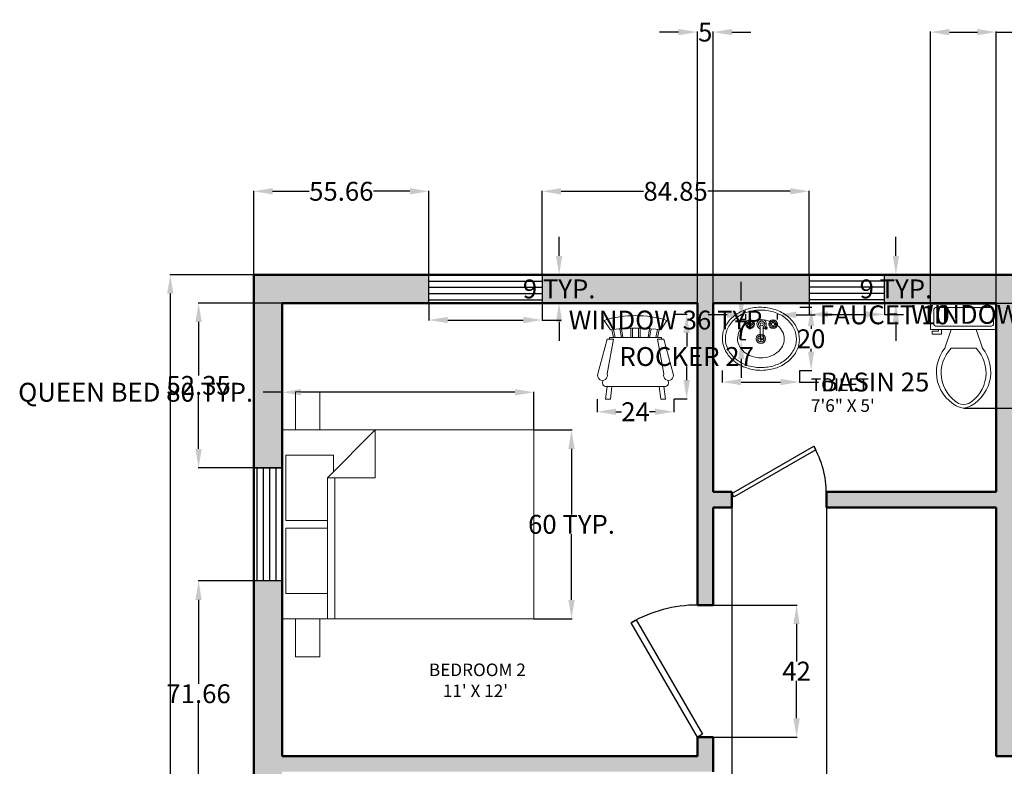
# Model space of a CAD drawing. Units: inches. Extents: x -40 to 482, y -490 to 102.
# Tile 3 of 4: x -40 to 273, y -136 to 102. Entities that reach past the tile are written whole.
import ezdxf

# ---------------------------------------------------------------- set-up
doc = ezdxf.new("R2010")
doc.units = ezdxf.units.IN
doc.header["$MEASUREMENT"] = 0
for name, color, linetype, lineweight in [('A-ANNO-DIMS', 2, 'Continuous', 18), ('A-AREA-IDEN', 7, 'Continuous', 18), ('A-FLOR-FIXT', 9, 'Continuous', 18), ('A-FURN', 8, 'Continuous', 18), ('A-WALL', 7, 'Continuous', 50), ('A-WALL-PATT', 251, 'Continuous', 13), ('DOOR', 21, 'Continuous', 25), ('WINDOW', 151, 'Continuous', 25)]:
    doc.layers.add(name, color=color, linetype=linetype, lineweight=lineweight)
doc.styles.get("Standard").update_dxf_attribs({"font": 'arial.ttf'})
doc.dimstyles.get("Standard").update_dxf_attribs({"dimtxt": 6, "dimasz": 6, "dimexe": 0.18, "dimexo": 0.0625, "dimgap": 0.09, "dimtad": 0, "dimtih": 1, "dimtoh": 1, "dimdec": 3, "dimzin": 0, "dimdsep": 46, "dimlunit": 4, "dimtxsty": 'Standard', "dimcen": 0.09, "dimadec": 0, "dimazin": 0, "dimtfac": 1, "dimtdec": 3, "dimtofl": 0, "dimtmove": 0, "dimatfit": 3, "dimfxl": 1, "dimtolj": 1, "dimtzin": 0, "dimarcsym": 0})

# ---------------------------------------------------------------- blocks, each defined once
blk = doc.blocks.new('*U2')
for p, q in [((0, 0), (0, -6)), ((40, 0), (40, -6))]:
    blk.add_line(p, q)
blk.add_lwpolyline([(0, 0), (34.64, 20), (35.52, 18.48), (0.87, -1.52)], close=True)
blk.add_arc((0, 0), 40, 0, 30)
blk = doc.blocks.new('*U3')
for p, q in [((-40, 0), (-40, 6)), ((0, 0), (0, 6))]:
    blk.add_line(p, q)
blk.add_lwpolyline([(0, 0), (-34.64, -20), (-35.52, -18.48), (-0.88, 1.52)], close=True)
blk.add_arc((0, 0), 40, 180, 210)
blk = doc.blocks.new('WINDOW')
for p, q in [((0, 0), (36, 0)), ((0, -9), (0, 0)), ((36, 0), (36, -9)), ((0, -2), (36, -2)), ((0, -4), (36, -4)), ((0, -6), (36, -6)), ((0, -8), (36, -8)), ((36, -9), (0, -9))]:
    blk.add_line(p, q)
blk = doc.blocks.new('Bed - Queen')
for p, q in [((0, -80.00003), (0, 0)), ((0, 0), (59.99999, 0)), ((59.99999, 0), (59.99999, -80.00003)), ((7.99999, -1.2), (28.79998, -1.2)), ((7.99999, -14.4), (7.99999, -1.2)), ((28.79998, -1.2), (28.79998, -14.4)), ((31.19999, -1.2), (51.99999, -1.2)), ((31.19999, -14.4), (31.19999, -1.2)), ((51.99999, -1.2), (51.99999, -16.4)), ((0, -14.4), (44.8, -14.4)), ((59.99999, -29.6), (44.8, -14.4)), ((44.8, -14.4), (44.8, -29.6)), ((44.8, -16.8), (0, -16.8)), ((51.99999, -16.4), (46.79936, -16.4)), ((44.8, -29.6), (59.99999, -29.6)), ((59.99999, -80.00003), (0, -80.00003))]:
    blk.add_line(p, q)
blk = doc.blocks.new('*U13')
for p, q in [((9.5, -6), (9.5, -2)), ((-10, -8.5), (-8, -8.5)), ((-10, -9.5), (-10, -8.5)), ((-8, -8.5), (-8, -8)), ((-7, -8), (-7, -9.5)), ((-4, -8), (-6, -14)), ((4, -8), (6, -14)), ((-7, -9.5), (-10, -9.5)), ((4, -14), (-4, -14))]:
    blk.add_line(p, q)
blk.add_lwpolyline([(10.5, -8), (10.5, 0), (-10.5, 0), (-10.5, -8)], close=True)
for points in [[(-9.5, -2), (-9.5, -6)], [(8.5, -1), (-8.5, -1)], [(-8.5, -7), (8.5, -7)]]:
    blk.add_lwpolyline(points)
for centre, radius, start, end in [((-8.62, -1.88), 0.884, 81.8699, 188.1301), ((8.62, -1.88), 0.884, 351.8699, 98.1301), ((-8.62, -6.12), 0.884, 171.8699, 278.1301), ((8.62, -6.12), 0.884, 261.8699, 8.1301), ((3.52, -21.58), 12.17, 141.4691, 247.9714), ((4.2, -21.82), 11.33, 136.3677, 238.9468), ((-3.52, -21.58), 12.17, 292.0284, 38.5307), ((-4.2, -21.82), 11.33, 301.053, 43.6321), ((0, -27.88), 4, 245.7318, 294.2682), ((0, -29), 4, 254.8605, 285.1395)]:
    blk.add_arc(centre, radius, start, end)
blk = doc.blocks.new('Chair - Rocking')
for p, q in [((-8, -4.5), (-10, -1.5)), ((8, -4.5), (10, -1.5)), ((-7.5, -4.5), (-7, -7)), ((-6.5, -7), (-7.02225, -4.43)), ((-4.5, -7), (-4.96674, -4.19951)), ((-4, -7), (-4.40532, -4.16272)), ((-1.5, -4.05012), (-1.5, -7)), ((-1, -7), (-1, -4.05012)), ((1, -7), (1, -4.04655)), ((1.5, -4.05012), (1.5, -7)), ((4, -7), (4.40187, -4.18694)), ((4.5, -7), (4.96761, -4.19437)), ((6.5, -7), (7, -4.4057)), ((7.5, -4.5), (7, -7)), ((-9, -7.5), (-12, -18.49999)), ((-7, -7.5), (-9, -7.5)), ((-9, -18.49999), (-7, -7.5)), ((-8.23428, -6.99939), (-8.3093, -7.47958)), ((-8.23041, -7), (8.23915, -7)), ((7, -7.5), (9, -7.5)), ((9, -18.49999), (7, -7.5)), ((8.31071, -7.48854), (8.23449, -7.00073)), ((9, -7.5), (12, -18.49999)), ((-10.36644, -20.64523), (-10.5, -21.49999)), ((10.5, -21.49999), (10.3575, -20.58798)), ((-9, -22.49999), (-9.5, -26.49999)), ((0, -22.49999), (-9.5, -22.49999)), ((-8, -26.49999), (-7.5, -22.49999)), ((0, -22.49999), (9.5, -22.49999)), ((8, -26.49999), (7.5, -22.49999)), ((9, -22.49999), (9.5, -26.49999)), ((-9.5, -26.49999), (-8, -26.49999)), ((9.5, -26.49999), (8, -26.49999))]:
    blk.add_line(p, q)
for centre, radius, start, end in [((0, -34.08333), 34.08333, 72.93847, 107.0615), ((0, -68.25004), 64.25, 93.92211, 97.15267), ((0, -68.25004), 64.25, 82.84733, 93.92211), ((-10.5, -18.99999), 1.58114, 161.5651, 18.43495), ((10.5, -18.99999), 1.58114, 161.5651, 18.43495), ((-9.5, -21.49999), 1, 180, 270), ((9.5, -21.49999), 1, 270, 0)]:
    blk.add_arc(centre, radius, start, end)
blk = doc.blocks.new('Sink - Oval top')
for p, q in [((-1, 0), (1, 0)), ((0, 1), (0, -1))]:
    blk.add_line(p, q)
for points in [[(-12.23, 0.39, 0.117634), (-11.46, -3.36, 0.104469), (-8.88, -6.8, 0.090016), (-5.08, -9.07, 0.08192), (-0.32, -10.02, 0.08192), (4.49, -9.38, 0.090016), (8.42, -7.36, 0.104469), (11.22, -4.09, 0.117634), (12.23, -0.39, 0.117634), (11.46, 3.36, 0.104469), (8.88, 6.8, 0.090016), (5.08, 9.07, 0.08192), (0.32, 10.02, 0.08192), (-4.49, 9.38, 0.090016), (-8.42, 7.36, 0.104469), (-11.22, 4.09, 0.117634)], [(-11.29, 0.16, 0.118622), (-10.52, -3.25, 0.104678), (-8.07, -6.36, 0.089562), (-4.54, -8.37, 0.081185), (-0.13, -9.15, 0.081185), (4.3, -8.49, 0.089562), (7.89, -6.58, 0.104678), (10.42, -3.55, 0.118622), (11.29, -0.16, 0.118622), (10.52, 3.25, 0.104678), (8.07, 6.36, 0.089562), (4.54, 8.37, 0.081185), (0.13, 9.15, 0.081185), (-4.3, 8.49, 0.089562), (-7.89, 6.58, 0.104678), (-10.42, 3.55, 0.118622)], [(-7.42, 0.08, 0.118283), (-6.91, -2.17, 0.104607), (-5.29, -4.21, 0.089718), (-2.97, -5.53, 0.081436), (-0.07, -6.04, 0.081436), (2.84, -5.59, 0.089718), (5.2, -4.33, 0.104607), (6.86, -2.32, 0.118283), (7.42, -0.08, 0.118283), (6.91, 2.17, 0.104607), (5.29, 4.21, 0.089718), (2.97, 5.53, 0.081436), (0.07, 6.04, 0.081436), (-2.84, 5.59, 0.089718), (-5.2, 4.33, 0.104607), (-6.86, 2.32, 0.118283)]]:
    blk.add_lwpolyline(points, format="xyb", close=True)
for radius in [1.5, 1]:
    blk.add_circle((0, 0), radius)
blk = doc.blocks.new('Faucet - Bathroom top')
for p, q in [((-4.107, 0.125), (-4.375, 0.125)), ((-3.75, 0.4788), (-3.75, 0.75)), ((-3.5, 0.482), (-3.5, 0.75)), ((-3.1461, 0.125), (-2.875, 0.125)), ((3.143, 0.125), (2.875, 0.125)), ((3.5, 0.4788), (3.5, 0.75)), ((3.75, 0.482), (3.75, 0.75)), ((4.1039, 0.125), (4.375, 0.125)), ((-4.1039, -0.125), (-4.375, -0.125)), ((-3.75, -0.4821), (-3.75, -0.75)), ((-3.5, -0.4789), (-3.5, -0.75)), ((-3.143, -0.125), (-2.875, -0.125)), ((-0.5, -0.8639), (-0.5, -4.5)), ((0.5, -4.5), (0.5, -0.8631)), ((3.1461, -0.125), (2.875, -0.125)), ((3.5, -0.4821), (3.5, -0.75)), ((3.75, -0.4789), (3.75, -0.75)), ((4.107, -0.125), (4.375, -0.125))]:
    blk.add_line(p, q)
for centre, radius in [((-3.625, 0), 1.375), ((-4.625, 0), 0.2795), ((-3.625, 0), 0.5), ((-3.625, 1), 0.2795), ((-2.625, 0), 0.2795), ((0, 0), 0.5), ((3.625, 0), 1.375), ((2.625, 0), 0.2795), ((3.625, 0), 0.5), ((3.625, 1), 0.2795), ((4.625, 0), 0.2795), ((-3.625, -1), 0.2795), ((3.625, -1), 0.2795)]:
    blk.add_circle(centre, radius)
for centre, radius, start, end in [((-3.625, 0), 1, 105.2407, 164.2093), ((-3.625, 0), 1, 16.44125, 74.07887), ((0, 0), 1.5, 289.6514, 250.3603), ((0, 0), 1, 300.3431, 239.7554), ((3.625, 0), 1, 106.12, 164.0884), ((3.625, 0), 1, 16.23422, 73.90469), ((-3.625, 0), 1, 196.2342, 253.9047), ((-3.625, 0), 1, 286.12, 344.0884), ((3.625, 0), 1, 196.4413, 254.0789), ((3.625, 0), 1, 285.2407, 344.2093), ((0, -4.5), 0.5, 180, 0)]:
    blk.add_arc(centre, radius, start, end)
blk = doc.blocks.new('WIN-24IN')
for p, q in [((24, 9), (0, 9)), ((0, 9), (0, 0)), ((24, 7), (0, 7)), ((24, 0), (24, 9)), ((24, 5), (0, 5)), ((24, 3), (0, 3)), ((24, 1), (0, 1)), ((0, 0), (24, 0))]:
    blk.add_line(p, q)
blk = doc.blocks.new('NIGHTSTAND')
blk.add_lwpolyline([(0, 12.15), (7.78, 12.15), (7.78, 0), (0, 0)], close=True)
blk = doc.blocks.new('*D24')
at = {"layer": 'A-ANNO-DIMS', "color": 0, "lineweight": -2, "transparency": 16777216}
for p, q in [((90.52, 11.43), (90.52, 5.91)), ((126.52, 11.43), (126.52, 5.91)), ((96.52, 6.09), (120.52, 6.09)), ((126.52, 6.09), (132.52, 6.09))]:
    blk.add_line(p, q, dxfattribs=at)
at = {"layer": 'A-ANNO-DIMS', "color": 0, "transparency": 16777216}
for points in [[(96.52, 7.09), (96.52, 5.09), (90.52, 6.09)], [(120.52, 7.09), (120.52, 5.09), (126.52, 6.09)]]:
    blk.add_solid(points, dxfattribs=at)
at = {"layer": 'Defpoints', "color": 0, "transparency": 16777216}
for p in [(90.52, 11.49), (126.52, 11.49), (126.52, 6.09)]:
    blk.add_point(p, dxfattribs=at)
at = {"layer": 'A-ANNO-DIMS', "color": 0, "transparency": 16777216, "insert": (166.89, 6.09), "char_height": 6, "attachment_point": 5}
blk.add_mtext('\\A1;WINDOW 36 TYP.', dxfattribs=at)
blk = doc.blocks.new('*D25')
at = {"layer": 'A-ANNO-DIMS', "color": 0, "lineweight": -2, "transparency": 16777216}
for p, q in [((131.92, 26.49), (131.92, 32.49)), ((126.58, 20.49), (132.1, 20.49)), ((126.58, 11.49), (132.1, 11.49)), ((131.92, 5.49), (131.92, -0.51))]:
    blk.add_line(p, q, dxfattribs=at)
at = {"layer": 'A-ANNO-DIMS', "color": 0, "transparency": 16777216}
for points in [[(130.92, 26.49), (132.92, 26.49), (131.92, 20.49)], [(130.92, 5.49), (132.92, 5.49), (131.92, 11.49)]]:
    blk.add_solid(points, dxfattribs=at)
at = {"layer": 'Defpoints', "color": 0, "transparency": 16777216}
for p in [(126.52, 20.49), (131.92, 20.49), (126.52, 11.49)]:
    blk.add_point(p, dxfattribs=at)
at = {"layer": 'A-ANNO-DIMS', "color": 0, "transparency": 16777216, "insert": (131.92, 15.99), "char_height": 6, "attachment_point": 5}
blk.add_mtext('\\A1;9 TYP.', dxfattribs=at)
blk = doc.blocks.new('*D26')
at = {"layer": 'A-ANNO-DIMS', "color": 0, "lineweight": -2, "transparency": 16777216}
for p, q in [((211.37, 11.43), (211.37, 7.71)), ((235.37, 11.43), (235.37, 7.71)), ((217.37, 7.89), (229.37, 7.89)), ((235.37, 7.89), (241.37, 7.89))]:
    blk.add_line(p, q, dxfattribs=at)
at = {"layer": 'A-ANNO-DIMS', "color": 0, "transparency": 16777216}
for points in [[(217.37, 8.89), (217.37, 6.89), (211.37, 7.89)], [(229.37, 8.89), (229.37, 6.89), (235.37, 7.89)]]:
    blk.add_solid(points, dxfattribs=at)
at = {"layer": 'Defpoints', "color": 0, "transparency": 16777216}
for p in [(211.37, 11.49), (235.37, 11.49), (235.37, 7.89)]:
    blk.add_point(p, dxfattribs=at)
at = {"layer": 'A-ANNO-DIMS', "color": 0, "transparency": 16777216, "insert": (275.73, 7.89), "char_height": 6, "attachment_point": 5}
blk.add_mtext('\\A1;WINDOW 24 TYP.', dxfattribs=at)
blk = doc.blocks.new('*D27')
at = {"layer": 'A-ANNO-DIMS', "color": 0, "lineweight": -2, "transparency": 16777216}
for p, q in [((238.97, 26.49), (238.97, 32.49)), ((235.43, 20.49), (239.15, 20.49)), ((235.43, 11.49), (239.15, 11.49)), ((238.97, 5.49), (238.97, -0.51))]:
    blk.add_line(p, q, dxfattribs=at)
at = {"layer": 'A-ANNO-DIMS', "color": 0, "transparency": 16777216}
for points in [[(237.97, 26.49), (239.97, 26.49), (238.97, 20.49)], [(237.97, 5.49), (239.97, 5.49), (238.97, 11.49)]]:
    blk.add_solid(points, dxfattribs=at)
at = {"layer": 'Defpoints', "color": 0, "transparency": 16777216}
for p in [(235.37, 20.49), (238.97, 20.49), (235.37, 11.49)]:
    blk.add_point(p, dxfattribs=at)
at = {"layer": 'A-ANNO-DIMS', "color": 0, "transparency": 16777216, "insert": (238.97, 15.99), "char_height": 6, "attachment_point": 5}
blk.add_mtext('\\A1;9 TYP.', dxfattribs=at)
blk = doc.blocks.new('*D32')
at = {"layer": 'A-ANNO-DIMS', "color": 0, "lineweight": -2, "transparency": 16777216}
for p, q in [((43.86, -16.86), (37.86, -16.86)), ((43.86, -28.8), (43.86, -16.68)), ((117.86, -16.86), (49.86, -16.86)), ((123.86, -28.8), (123.86, -16.68))]:
    blk.add_line(p, q, dxfattribs=at)
at = {"layer": 'A-ANNO-DIMS', "color": 0, "transparency": 16777216}
for points in [[(49.86, -15.86), (49.86, -17.86), (43.86, -16.86)], [(117.86, -15.86), (117.86, -17.86), (123.86, -16.86)]]:
    blk.add_solid(points, dxfattribs=at)
at = {"layer": 'Defpoints', "color": 0, "transparency": 16777216}
for p in [(43.86, -16.86), (43.86, -28.86), (123.86, -28.86)]:
    blk.add_point(p, dxfattribs=at)
at = {"layer": 'A-ANNO-DIMS', "color": 0, "transparency": 16777216, "insert": (-2.68, -16.86), "char_height": 6, "attachment_point": 5}
blk.add_mtext('\\A1;QUEEN BED 80 TYP.', dxfattribs=at)
blk = doc.blocks.new('*D33')
at = {"layer": 'A-ANNO-DIMS', "color": 0, "lineweight": -2, "transparency": 16777216}
for p, q in [((123.92, -28.86), (136.04, -28.86)), ((135.86, -34.86), (135.86, -55.71)), ((135.86, -82.86), (135.86, -62.02)), ((123.92, -88.86), (136.04, -88.86))]:
    blk.add_line(p, q, dxfattribs=at)
at = {"layer": 'A-ANNO-DIMS', "color": 0, "transparency": 16777216}
for points in [[(134.86, -34.86), (136.86, -34.86), (135.86, -28.86)], [(134.86, -82.86), (136.86, -82.86), (135.86, -88.86)]]:
    blk.add_solid(points, dxfattribs=at)
at = {"layer": 'Defpoints', "color": 0, "transparency": 16777216}
for p in [(123.86, -28.86), (135.86, -28.86), (123.86, -88.86)]:
    blk.add_point(p, dxfattribs=at)
at = {"layer": 'A-ANNO-DIMS', "color": 0, "transparency": 16777216, "insert": (135.86, -58.86), "char_height": 6, "attachment_point": 5}
blk.add_mtext('\\A1;60 TYP.', dxfattribs=at)
blk = doc.blocks.new('*D36')
at = {"layer": 'A-ANNO-DIMS', "color": 0, "lineweight": -2, "transparency": 16777216}
for p, q in [((168.48, 7.99), (172.64, 7.99)), ((172.46, 1.99), (172.46, -2.32)), ((172.46, -13.01), (172.46, -8.71)), ((168.48, -19.01), (172.64, -19.01))]:
    blk.add_line(p, q, dxfattribs=at)
at = {"layer": 'A-ANNO-DIMS', "color": 0, "transparency": 16777216}
for points in [[(171.46, 1.99), (173.46, 1.99), (172.46, 7.99)], [(171.46, -13.01), (173.46, -13.01), (172.46, -19.01)]]:
    blk.add_solid(points, dxfattribs=at)
at = {"layer": 'Defpoints', "color": 0, "transparency": 16777216}
for p in [(168.41, 7.99), (172.46, 7.99), (168.41, -19.01)]:
    blk.add_point(p, dxfattribs=at)
at = {"layer": 'A-ANNO-DIMS', "color": 0, "transparency": 16777216, "insert": (172.46, -5.51), "char_height": 6, "attachment_point": 5}
blk.add_mtext('\\A1;ROCKER 27', dxfattribs=at)
blk = doc.blocks.new('*D37')
at = {"layer": 'A-ANNO-DIMS', "color": 0, "lineweight": -2, "transparency": 16777216}
for p, q in [((143.98, -19.07), (143.98, -23.24)), ((168.41, -19.07), (168.41, -23.24)), ((149.98, -23.06), (151.77, -23.06)), ((162.41, -23.06), (160.62, -23.06))]:
    blk.add_line(p, q, dxfattribs=at)
at = {"layer": 'A-ANNO-DIMS', "color": 0, "transparency": 16777216}
for points in [[(149.98, -22.06), (149.98, -24.06), (143.98, -23.06)], [(162.41, -22.06), (162.41, -24.06), (168.41, -23.06)]]:
    blk.add_solid(points, dxfattribs=at)
at = {"layer": 'Defpoints', "color": 0, "transparency": 16777216}
for p in [(143.98, -19.01), (168.41, -19.01), (168.41, -23.06)]:
    blk.add_point(p, dxfattribs=at)
at = {"layer": 'A-ANNO-DIMS', "color": 0, "transparency": 16777216, "insert": (156.2, -23.06), "char_height": 6, "attachment_point": 5}
blk.add_mtext('\\A1;24', dxfattribs=at)
blk = doc.blocks.new('*D38')
at = {"layer": 'A-ANNO-DIMS', "color": 0, "lineweight": -2, "transparency": 16777216}
for p, q in [((183.77, -10), (183.77, -13.8)), ((208.33, -10), (208.33, -13.8)), ((189.77, -13.62), (202.33, -13.62)), ((208.33, -13.62), (214.33, -13.62))]:
    blk.add_line(p, q, dxfattribs=at)
at = {"layer": 'A-ANNO-DIMS', "color": 0, "transparency": 16777216}
for points in [[(189.77, -12.62), (189.77, -14.62), (183.77, -13.62)], [(202.33, -12.62), (202.33, -14.62), (208.33, -13.62)]]:
    blk.add_solid(points, dxfattribs=at)
at = {"layer": 'Defpoints', "color": 0, "transparency": 16777216}
for p in [(183.77, -9.94), (208.33, -9.94), (208.33, -13.62)]:
    blk.add_point(p, dxfattribs=at)
at = {"layer": 'A-ANNO-DIMS', "color": 0, "transparency": 16777216, "insert": (232.34, -13.62), "char_height": 6, "attachment_point": 5}
blk.add_mtext('\\A1;BASIN 25', dxfattribs=at)
blk = doc.blocks.new('*D39')
at = {"layer": 'A-ANNO-DIMS', "color": 0, "lineweight": -2, "transparency": 16777216}
for p, q in [((208.39, 10.2), (212.19, 10.2)), ((212.01, 4.2), (212.01, 3.28)), ((212.01, -3.94), (212.01, -3.03)), ((208.39, -9.94), (212.19, -9.94))]:
    blk.add_line(p, q, dxfattribs=at)
at = {"layer": 'A-ANNO-DIMS', "color": 0, "transparency": 16777216}
for points in [[(211.01, 4.2), (213.01, 4.2), (212.01, 10.2)], [(211.01, -3.94), (213.01, -3.94), (212.01, -9.94)]]:
    blk.add_solid(points, dxfattribs=at)
at = {"layer": 'Defpoints', "color": 0, "transparency": 16777216}
for p in [(208.33, 10.2), (212.01, 10.2), (208.33, -9.94)]:
    blk.add_point(p, dxfattribs=at)
at = {"layer": 'A-ANNO-DIMS', "color": 0, "transparency": 16777216, "insert": (212.01, 0.13), "char_height": 6, "attachment_point": 5}
blk.add_mtext('\\A1;20', dxfattribs=at)
blk = doc.blocks.new('*D40')
at = {"layer": 'A-ANNO-DIMS', "color": 0, "lineweight": -2, "transparency": 16777216}
for p, q in [((185.29, 7.75), (179.29, 7.75)), ((191.29, 6.31), (191.29, 7.93)), ((201.29, 6.31), (201.29, 7.93)), ((207.29, 7.75), (213.29, 7.75))]:
    blk.add_line(p, q, dxfattribs=at)
at = {"layer": 'A-ANNO-DIMS', "color": 0, "transparency": 16777216}
for points in [[(185.29, 8.75), (185.29, 6.75), (191.29, 7.75)], [(207.29, 8.75), (207.29, 6.75), (201.29, 7.75)]]:
    blk.add_solid(points, dxfattribs=at)
at = {"layer": 'Defpoints', "color": 0, "transparency": 16777216}
for p in [(201.29, 7.75), (191.29, 6.25), (201.29, 6.25)]:
    blk.add_point(p, dxfattribs=at)
at = {"layer": 'A-ANNO-DIMS', "color": 0, "transparency": 16777216, "insert": (235.42, 7.75), "char_height": 6, "attachment_point": 5}
blk.add_mtext('\\A1;FAUCET 10', dxfattribs=at)
blk = doc.blocks.new('*D41')
at = {"layer": 'A-ANNO-DIMS', "color": 0, "lineweight": -2, "transparency": 16777216}
for p, q in [((189.79, 12.25), (189.79, 18.25)), ((191.23, 6.25), (189.61, 6.25)), ((191.23, -0.25), (189.61, -0.25)), ((189.79, -6.25), (189.79, -12.25))]:
    blk.add_line(p, q, dxfattribs=at)
at = {"layer": 'A-ANNO-DIMS', "color": 0, "transparency": 16777216}
for points in [[(188.79, 12.25), (190.79, 12.25), (189.79, 6.25)], [(188.79, -6.25), (190.79, -6.25), (189.79, -0.25)]]:
    blk.add_solid(points, dxfattribs=at)
at = {"layer": 'Defpoints', "color": 0, "transparency": 16777216}
for p in [(189.79, 6.25), (191.29, 6.25), (191.29, -0.25)]:
    blk.add_point(p, dxfattribs=at)
at = {"layer": 'A-ANNO-DIMS', "color": 0, "transparency": 16777216, "insert": (189.79, 3), "char_height": 6, "attachment_point": 5}
blk.add_mtext('\\A1;7', dxfattribs=at)
blk = doc.blocks.new('*D53')
at = {"layer": 'A-ANNO-DIMS', "color": 0, "lineweight": -2, "transparency": 16777216}
for p, q in [((34.79, 20.49), (8.14, 20.49)), ((8.32, 14.49), (8.32, -216.36)), ((8.32, -453.51), (8.32, -222.66)), ((34.79, -459.51), (8.14, -459.51))]:
    blk.add_line(p, q, dxfattribs=at)
at = {"layer": 'A-ANNO-DIMS', "color": 0, "transparency": 16777216}
for points in [[(7.32, 14.49), (9.32, 14.49), (8.32, 20.49)], [(7.32, -453.51), (9.32, -453.51), (8.32, -459.51)]]:
    blk.add_solid(points, dxfattribs=at)
at = {"layer": 'Defpoints', "color": 0, "transparency": 16777216}
for p in [(8.32, 20.49), (34.86, 20.49), (34.86, -459.51)]:
    blk.add_point(p, dxfattribs=at)
at = {"layer": 'A-ANNO-DIMS', "color": 0, "transparency": 16777216, "insert": (8.32, -219.51), "char_height": 6, "attachment_point": 5}
blk.add_mtext('\\A1;480', dxfattribs=at)
blk = doc.blocks.new('*D54')
at = {"layer": 'A-ANNO-DIMS', "color": 0, "lineweight": -2, "transparency": 16777216}
for p, q in [((34.86, 20.55), (34.86, 47.2)), ((40.86, 47.02), (52.48, 47.02)), ((84.52, 47.02), (72.9, 47.02)), ((90.52, 20.55), (90.52, 47.2))]:
    blk.add_line(p, q, dxfattribs=at)
at = {"layer": 'A-ANNO-DIMS', "color": 0, "transparency": 16777216}
for points in [[(40.86, 48.02), (40.86, 46.02), (34.86, 47.02)], [(84.52, 48.02), (84.52, 46.02), (90.52, 47.02)]]:
    blk.add_solid(points, dxfattribs=at)
at = {"layer": 'Defpoints', "color": 0, "transparency": 16777216}
for p in [(90.52, 47.02), (34.86, 20.49), (90.52, 20.49)]:
    blk.add_point(p, dxfattribs=at)
at = {"layer": 'A-ANNO-DIMS', "color": 0, "transparency": 16777216, "insert": (62.69, 47.02), "char_height": 6, "attachment_point": 5}
blk.add_mtext('\\A1;55.66', dxfattribs=at)
blk = doc.blocks.new('*D55')
at = {"layer": 'A-ANNO-DIMS', "color": 0, "lineweight": -2, "transparency": 16777216}
for p, q in [((126.52, 20.55), (126.52, 47.2)), ((132.52, 47.02), (158.7, 47.02)), ((205.37, 47.02), (179.18, 47.02)), ((211.37, 20.55), (211.37, 47.2))]:
    blk.add_line(p, q, dxfattribs=at)
at = {"layer": 'A-ANNO-DIMS', "color": 0, "transparency": 16777216}
for points in [[(132.52, 48.02), (132.52, 46.02), (126.52, 47.02)], [(205.37, 48.02), (205.37, 46.02), (211.37, 47.02)]]:
    blk.add_solid(points, dxfattribs=at)
at = {"layer": 'Defpoints', "color": 0, "transparency": 16777216}
for p in [(211.37, 47.02), (126.52, 20.49), (211.37, 20.49)]:
    blk.add_point(p, dxfattribs=at)
at = {"layer": 'A-ANNO-DIMS', "color": 0, "transparency": 16777216, "insert": (168.94, 47.02), "char_height": 6, "attachment_point": 5}
blk.add_mtext('\\A1;84.85', dxfattribs=at)
blk = doc.blocks.new('*D56')
at = {"layer": 'A-ANNO-DIMS', "color": 0, "lineweight": -2, "transparency": 16777216}
for p, q in [((43.79, 11.49), (17.14, 11.49)), ((17.32, 5.49), (17.32, -11.53)), ((17.32, -34.86), (17.32, -17.84)), ((43.79, -40.86), (17.14, -40.86))]:
    blk.add_line(p, q, dxfattribs=at)
at = {"layer": 'A-ANNO-DIMS', "color": 0, "transparency": 16777216}
for points in [[(16.32, 5.49), (18.32, 5.49), (17.32, 11.49)], [(16.32, -34.86), (18.32, -34.86), (17.32, -40.86)]]:
    blk.add_solid(points, dxfattribs=at)
at = {"layer": 'Defpoints', "color": 0, "transparency": 16777216}
for p in [(17.32, 11.49), (43.86, 11.49), (43.86, -40.86)]:
    blk.add_point(p, dxfattribs=at)
at = {"layer": 'A-ANNO-DIMS', "color": 0, "transparency": 16777216, "insert": (17.32, -14.69), "char_height": 6, "attachment_point": 5}
blk.add_mtext('\\A1;52.35', dxfattribs=at)
blk = doc.blocks.new('*D57')
at = {"layer": 'A-ANNO-DIMS', "color": 0, "lineweight": -2, "transparency": 16777216}
for p, q in [((43.79, -76.86), (17.14, -76.86)), ((17.32, -82.86), (17.32, -109.54)), ((17.32, -142.52), (17.32, -115.84)), ((43.79, -148.52), (17.14, -148.52))]:
    blk.add_line(p, q, dxfattribs=at)
at = {"layer": 'A-ANNO-DIMS', "color": 0, "transparency": 16777216}
for points in [[(16.32, -82.86), (18.32, -82.86), (17.32, -76.86)], [(16.32, -142.52), (18.32, -142.52), (17.32, -148.52)]]:
    blk.add_solid(points, dxfattribs=at)
at = {"layer": 'Defpoints', "color": 0, "transparency": 16777216}
for p in [(17.32, -76.86), (43.86, -76.86), (43.86, -148.52)]:
    blk.add_point(p, dxfattribs=at)
at = {"layer": 'A-ANNO-DIMS', "color": 0, "transparency": 16777216, "insert": (17.32, -112.69), "char_height": 6, "attachment_point": 5}
blk.add_mtext('\\A1;71.66', dxfattribs=at)
blk = doc.blocks.new('*D63')
at = {"layer": 'A-ANNO-DIMS', "color": 0, "lineweight": -2, "transparency": 16777216}
for p, q in [((186.86, -53.57), (186.86, -486.22)), ((216.86, -53.57), (216.86, -486.22)), ((192.86, -486.04), (197.48, -486.04)), ((210.86, -486.04), (206.23, -486.04))]:
    blk.add_line(p, q, dxfattribs=at)
at = {"layer": 'A-ANNO-DIMS', "color": 0, "transparency": 16777216}
for points in [[(192.86, -485.04), (192.86, -487.04), (186.86, -486.04)], [(210.86, -485.04), (210.86, -487.04), (216.86, -486.04)]]:
    blk.add_solid(points, dxfattribs=at)
at = {"layer": 'Defpoints', "color": 0, "transparency": 16777216}
for p in [(186.86, -53.51), (216.86, -53.51), (216.86, -486.04)]:
    blk.add_point(p, dxfattribs=at)
at = {"layer": 'A-ANNO-DIMS', "color": 0, "transparency": 16777216, "insert": (201.86, -486.04), "char_height": 6, "attachment_point": 5}
blk.add_mtext('\\A1;30', dxfattribs=at)
blk = doc.blocks.new('*D68')
at = {"layer": 'A-ANNO-DIMS', "color": 0, "lineweight": -2, "transparency": 16777216}
for p, q in [((249.98, 11.16), (249.98, 97.81)), ((255.98, 97.63), (264.86, 97.63)), ((270.86, 11.55), (270.86, 97.81)), ((270.86, 97.63), (276.86, 97.63))]:
    blk.add_line(p, q, dxfattribs=at)
at = {"layer": 'A-ANNO-DIMS', "color": 0, "transparency": 16777216}
for points in [[(255.98, 98.63), (255.98, 96.63), (249.98, 97.63)], [(264.86, 98.63), (264.86, 96.63), (270.86, 97.63)]]:
    blk.add_solid(points, dxfattribs=at)
at = {"layer": 'Defpoints', "color": 0, "transparency": 16777216}
for p in [(270.86, 97.63), (249.98, 11.1), (270.86, 11.49)]:
    blk.add_point(p, dxfattribs=at)
at = {"layer": 'A-ANNO-DIMS', "color": 0, "transparency": 16777216, "insert": (289.45, 97.63), "char_height": 6, "attachment_point": 5}
blk.add_mtext('\\A1;20.876', dxfattribs=at)
blk = doc.blocks.new('*D69')
at = {"layer": 'A-ANNO-DIMS', "color": 0, "lineweight": -2, "transparency": 16777216}
for p, q in [((270.92, 11.49), (471.86, 11.49)), ((471.68, 5.49), (471.68, -2.05)), ((471.68, -15.9), (471.68, -8.36)), ((260.54, -21.9), (471.86, -21.9))]:
    blk.add_line(p, q, dxfattribs=at)
at = {"layer": 'A-ANNO-DIMS', "color": 0, "transparency": 16777216}
for points in [[(470.68, 5.49), (472.68, 5.49), (471.68, 11.49)], [(470.68, -15.9), (472.68, -15.9), (471.68, -21.9)]]:
    blk.add_solid(points, dxfattribs=at)
at = {"layer": 'Defpoints', "color": 0, "transparency": 16777216}
for p in [(270.86, 11.49), (471.68, 11.49), (260.48, -21.9)]:
    blk.add_point(p, dxfattribs=at)
at = {"layer": 'A-ANNO-DIMS', "color": 0, "transparency": 16777216, "insert": (471.68, -5.2), "char_height": 6, "attachment_point": 5}
blk.add_mtext('\\A1;33.39', dxfattribs=at)
blk = doc.blocks.new('*D70')
at = {"layer": 'A-ANNO-DIMS', "color": 0, "lineweight": -2, "transparency": 16777216}
for p, q in [((169.855436, 97.632056), (163.855436, 97.632056)), ((175.855436, 11.553413), (175.855436, 97.812056)), ((180.855436, 11.553413), (180.855436, 97.812056)), ((186.855436, 97.632056), (192.855436, 97.632056))]:
    blk.add_line(p, q, dxfattribs=at)
at = {"layer": 'A-ANNO-DIMS', "color": 0, "transparency": 16777216}
for points in [[(169.855436, 98.632056), (169.855436, 96.632056), (175.855436, 97.632056)], [(186.855436, 98.632056), (186.855436, 96.632056), (180.855436, 97.632056)]]:
    blk.add_solid(points, dxfattribs=at)
at = {"layer": 'Defpoints', "color": 0, "transparency": 16777216}
for p in [(180.855436, 97.632056), (175.855436, 11.490913), (180.855436, 11.490913)]:
    blk.add_point(p, dxfattribs=at)
at = {"layer": 'A-ANNO-DIMS', "color": 0, "transparency": 16777216, "insert": (178.355436, 97.632056), "char_height": 6, "attachment_point": 5}
blk.add_mtext('\\A1;5', dxfattribs=at)
blk = doc.blocks.new('*D74')
at = {"layer": 'A-ANNO-DIMS', "color": 0, "lineweight": -2, "transparency": 16777216}
for p, q in [((180.92, -84.51), (207.57, -84.51)), ((207.39, -90.51), (207.39, -102.41)), ((207.39, -120.51), (207.39, -108.61)), ((180.92, -126.51), (207.57, -126.51))]:
    blk.add_line(p, q, dxfattribs=at)
at = {"layer": 'A-ANNO-DIMS', "color": 0, "transparency": 16777216}
for points in [[(206.39, -90.51), (208.39, -90.51), (207.39, -84.51)], [(206.39, -120.51), (208.39, -120.51), (207.39, -126.51)]]:
    blk.add_solid(points, dxfattribs=at)
at = {"layer": 'Defpoints', "color": 0, "transparency": 16777216}
for p in [(180.86, -84.51), (180.86, -126.51), (207.39, -126.51)]:
    blk.add_point(p, dxfattribs=at)
at = {"layer": 'A-ANNO-DIMS', "color": 0, "transparency": 16777216, "insert": (207.39, -105.51), "char_height": 6, "attachment_point": 5}
blk.add_mtext('\\A1;42', dxfattribs=at)

msp = doc.modelspace()

# ---------------------------------------------------------------- hatches: boundary and pattern name
at = {"layer": 'A-WALL-PATT'}
h = msp.add_hatch(color=256, dxfattribs=at)
h.dxf.hatch_style = 1
h.paths.add_polyline_path([(394.8554, -267.0722), (385.8554, -267.0722), (385.8554, -280.5091), (361.8554, -280.5091), (361.8554, -285.5091), (385.8554, -285.5091), (385.8554, -344.9426), (394.8554, -344.9426)])
h.paths.add_polyline_path([(394.8554, -171.3545), (385.8554, -171.3545), (385.8554, -185.5091), (325.8554, -185.5091), (325.8554, -173.5091), (320.8554, -173.5091), (320.8554, -190.5091), (320.8554, -277.5091), (295.8554, -277.5091), (295.8554, -282.5091), (320.8554, -282.5091), (320.8554, -285.5091), (331.8554, -285.5091), (331.8554, -280.5091), (325.8554, -280.5091), (325.8554, -190.5091), (386.1154, -190.5091), (386.1154, -226.6962), (386.0363, -243.0722), (394.8554, -243.0722)])
h.paths.add_polyline_path([(394.8554, -83.9679), (385.8554, -83.9679), (385.8554, -127.5091), (320.8554, -127.5091), (320.8554, -137.5091), (320.8554, -143.5091), (325.8554, -143.5091), (325.8554, -137.5091), (385.8554, -137.5091), (385.8554, -147.3545), (394.8554, -147.3545)])
h.paths.add_polyline_path([(394.8554, 20.4909), (235.3658, 20.4909), (235.3658, 11.4909), (270.8554, 11.4909), (270.9798, 11.1006), (270.9798, 3.1006), (270.8554, -48.5091), (216.8554, -48.5091), (216.8554, -53.5091), (270.8554, -53.5091), (270.8554, -132.5091), (275.8554, -132.5091), (275.8554, 11.4909), (311.8554, 11.4909), (385.8554, 11.4909), (385.8554, -47.9679), (394.8554, -47.9679)])
h.paths.add_polyline_path([(211.3658, 20.4909), (126.5194, 20.4909), (126.5194, 11.4909), (175.8554, 11.4909), (175.8554, -84.5091), (180.8554, -84.5091), (180.8554, -53.5091), (186.8554, -53.5091), (186.8554, -48.5091), (180.8554, -48.5091), (180.8554, 11.4909), (211.3658, 11.4909)])
h.paths.add_polyline_path([(90.5194, 20.4909), (34.8554, 20.4909), (34.8554, -40.8616), (43.8554, -40.8616), (43.8554, -28.8616), (43.8554, 11.4909), (90.5194, 11.4909)])
h.paths.add_polyline_path([(43.8554, -76.8616), (34.8554, -76.8616), (34.8554, -148.5194), (43.8554, -148.5194), (43.8554, -137.5091), (180.8554, -137.5091), (180.8554, -126.5091), (175.8554, -126.5091), (175.8554, -132.5091), (43.8554, -132.5091)])
h.paths.add_polyline_path([(171.3012, -209.5091), (43.8554, -209.5091), (43.8554, -184.5194), (34.8554, -184.5194), (34.8554, -251.068), (43.8554, -251.068), (43.8554, -244.7708), (43.8554, -214.5091), (166.3012, -214.5091), (166.3012, -220.5091), (171.3012, -220.5091)])
h.paths.add_polyline_path([(171.3012, -262.5091), (166.3012, -262.5091), (166.3012, -334.5091), (43.8554, -334.5091), (43.8554, -287.068), (34.8554, -287.068), (34.8554, -459.5091), (43.8554, -459.5091), (49.8554, -459.5091), (49.8554, -450.5091), (43.8554, -450.5091), (43.8554, -339.5091), (166.3012, -339.5091), (166.3012, -450.5091), (160.3012, -450.5091), (160.3012, -459.5091), (166.3012, -459.5091), (171.3012, -459.5091), (171.3012, -450.5091), (171.3012, -445.9382), (171.3012, -410.0635), (171.3012, -407.0635), (186.7114, -407.0635), (186.7114, -401.0635), (171.3012, -401.0635)])
h.paths.add_polyline_path([(394.8554, -380.9426), (385.8554, -380.9426), (385.8554, -450.5091), (247.8554, -450.5091), (247.8554, -282.5091), (253.8554, -282.5091), (253.8554, -277.5091), (242.8554, -277.5091), (242.8554, -401.0635), (228.7114, -401.0635), (228.7114, -407.0635), (242.8554, -407.0635), (242.8554, -410.0635), (242.8554, -419.0322), (242.8554, -450.5091), (242.8554, -454.9068), (242.8554, -459.5091), (394.8554, -459.5091)])

# ---------------------------------------------------------------- linework, layer by layer
at = {"layer": 'A-WALL'}
for p, q in [((43.8554, 11.4909), (175.8554, 11.4909)), ((43.8554, -132.5091), (43.8554, 11.4909)), ((175.8554, -84.5091), (175.8554, 11.4909)), ((180.8554, 11.4909), (270.8554, 11.4909)), ((180.8554, -48.5091), (180.8554, 11.4909)), ((270.8554, -48.5091), (270.8554, 11.4909)), ((180.8554, -48.5091), (186.8554, -48.5091)), ((186.8554, -48.5091), (186.8554, -53.5091)), ((216.8554, -48.5091), (216.8554, -53.5091)), ((216.8554, -48.5091), (270.8554, -48.5091)), ((180.8554, -53.5091), (186.8554, -53.5091)), ((180.8554, -84.5091), (180.8554, -53.5091)), ((216.8554, -53.5091), (270.8554, -53.5091)), ((270.8554, -132.5091), (270.8554, -53.5091)), ((175.8554, -84.5091), (180.8554, -84.5091)), ((175.8554, -132.5091), (175.8554, -126.5091)), ((175.8554, -126.5091), (180.8554, -126.5091)), ((180.8554, -137.5091), (180.8554, -126.5091)), ((43.8554, -132.5091), (175.8554, -132.5091)), ((270.8554, -132.5091), (275.8554, -132.5091))]:
    msp.add_line(p, q, dxfattribs=at)
msp.add_lwpolyline([(43.8554, -459.5091), (34.8554, -459.5091), (34.8554, 20.4909), (394.8554, 20.4909), (394.8554, -459.5091), (242.8554, -459.5091)], dxfattribs=at)

# ---------------------------------------------------------------- block references
at = {"layer": 'A-FLOR-FIXT'}
for name, p in [('Sink - Oval top', (196.0499, 0.1283)), ('*U13', (260.4798, 11.1006)), ('Faucet - Bathroom top', (196.2892, 4.7503))]:
    msp.add_blockref(name, p, dxfattribs=at)
at = {"layer": 'A-FURN'}
for name, p in [('Chair - Rocking', (156.1966, 7.4892)), ('NIGHTSTAND', (48.126, -28.862)), ('NIGHTSTAND', (48.126, -101.0158))]:
    msp.add_blockref(name, p, dxfattribs=at)
at = {"layer": 'A-FURN', "rotation": 90}
msp.add_blockref('Bed - Queen', (43.8554, -88.8616), dxfattribs=at)
at = {"layer": 'DOOR', "xscale": 0.75, "yscale": 0.75, "zscale": 0.75}
msp.add_blockref('*U2', (186.8554, -49.0091), dxfattribs=at)
at = {"layer": 'DOOR', "xscale": 1.05, "yscale": 1.05, "zscale": 1.05, "rotation": 270}
msp.add_blockref('*U3', (175.8554, -126.5091), dxfattribs=at)
at = {"layer": 'WINDOW'}
for name, p in [('WINDOW', (90.5194, 20.4909)), ('WIN-24IN', (211.366, 11.491))]:
    msp.add_blockref(name, p, dxfattribs=at)
at = {"layer": 'WINDOW', "rotation": 270}
msp.add_blockref('WINDOW', (43.8554, -40.8616), dxfattribs=at)

# ---------------------------------------------------------------- texts
at = {"layer": 'A-AREA-IDEN', "char_height": 4, "attachment_point": 1}
for s, width, insert in [('TOILET\\P7\'6" X 5\'', 38.747987, (211.9609, -12.4268)), ("\\pxqc; BEDROOM 2\\P11' X 12'", 79.218438, (65.7117, -103.1037))]:
    msp.add_mtext_dynamic_manual_height_columns(s, width=width, gutter_width=1, heights=[0], dxfattribs=dict(at, insert=insert))

# ---------------------------------------------------------------- dimensions: what is measured, and where the dimension line sits
at = {"layer": 'A-ANNO-DIMS'}
for base, p1, p2, override, picture, middle in [((180.8554, 97.6321), (175.8554, 11.4909), (180.8554, 11.4909), {"dimdec": 0, "dimlfac": 1, "dimrnd": 0, "dimzin": 0, "dimdsep": 46, "dimlunit": 2}, '*D70', (178.3554, 97.6321)), ((270.8554, 97.6321), (249.9798, 11.1006), (270.8554, 11.4909), {"dimdec": 3, "dimlfac": 1, "dimrnd": 0, "dimzin": 0, "dimdsep": 46, "dimlunit": 2}, '*D68', (289.4488, 97.6321)), ((90.5194, 47.0224), (34.8554, 20.4909), (90.5194, 20.4909), {"dimdec": 2, "dimlfac": 1, "dimrnd": 0, "dimzin": 0, "dimdsep": 46, "dimlunit": 2}, '*D54', (62.6874, 47.0224)), ((168.4142, -23.0608), (143.9791, -19.0108), (168.4142, -19.0108), {"dimdec": 0, "dimlfac": 1, "dimrnd": 0, "dimzin": 0, "dimdsep": 46, "dimlunit": 2}, '*D37', (156.1966, -23.0608)), ((216.8554, -486.0406), (186.8554, -53.5091), (216.8554, -53.5091), {"dimdec": 0, "dimlfac": 1, "dimrnd": 0, "dimzin": 0, "dimdsep": 46, "dimlunit": 2}, '*D63', (201.8554, -486.0406))]:
    dim = msp.add_linear_dim(base=base, p1=p1, p2=p2, dimstyle='Standard', override=override, dxfattribs=at)
    dim.commit()
    dim.dimension.update_dxf_attribs({"geometry": picture, "text_midpoint": middle})
for base, p1, p2, angle, override, picture, middle in [((211.3658, 47.0224), (126.5194, 20.4909), (211.3658, 20.4909), 0, {"dimdec": 2, "dimlfac": 1, "dimrnd": 0, "dimzin": 0, "dimdsep": 46, "dimlunit": 2}, '*D55', (168.9426, 47.0224)), ((8.3239, 20.4909), (34.8554, -459.5091), (34.8554, 20.4909), 90, {"dimdec": 0, "dimlfac": 1, "dimrnd": 0, "dimzin": 0, "dimdsep": 46, "dimlunit": 2}, '*D53', (8.3239, -219.5091)), ((189.7892, 6.2504), (191.2892, -0.2497), (191.2892, 6.2504), 90, {"dimdec": 0, "dimlfac": 1, "dimrnd": 0, "dimzin": 0, "dimdsep": 46, "dimlunit": 2}, '*D41', (189.7892, 3.0004)), ((17.3239, 11.4909), (43.8554, -40.8616), (43.8554, 11.4909), 90, {"dimdec": 2, "dimlfac": 1, "dimrnd": 0, "dimzin": 0, "dimdsep": 46, "dimlunit": 2}, '*D56', (17.3239, -14.6854)), ((212.008, 10.1965), (208.3254, -9.94), (208.3254, 10.1965), 90, {"dimdec": 0, "dimlfac": 1, "dimrnd": 0, "dimzin": 0, "dimdsep": 46, "dimlunit": 2}, '*D39', (212.008, 0.1283)), ((471.6767, 11.4909), (260.4799, -21.8994), (270.8554, 11.4909), 90, {"dimdec": 2, "dimlfac": 1, "dimrnd": 0, "dimzin": 0, "dimdsep": 46, "dimlunit": 2}, '*D69', (471.6767, -5.2042)), ((17.3239, -76.8616), (43.8554, -148.5194), (43.8554, -76.8616), 90, {"dimdec": 2, "dimlfac": 1, "dimrnd": 0, "dimzin": 0, "dimdsep": 46, "dimlunit": 2}, '*D57', (17.3239, -112.6905)), ((207.3869, -126.5091), (180.8554, -84.5091), (180.8554, -126.5091), 270, {"dimdec": 0, "dimlfac": 1, "dimrnd": 0, "dimzin": 0, "dimdsep": 46, "dimlunit": 2}, '*D74', (207.3869, -105.5091))]:
    dim = msp.add_linear_dim(base=base, p1=p1, p2=p2, angle=angle, dimstyle='Standard', override=override, dxfattribs=at)
    dim.commit()
    dim.dimension.update_dxf_attribs({"geometry": picture, "text_midpoint": middle})
for base, p1, p2, angle, text, picture, middle in [((131.9194, 20.4909), (126.5194, 11.4909), (126.5194, 20.4909), 90, '<> TYP.', '*D25', (131.9194, 15.9909)), ((238.9658, 20.4909), (235.3658, 11.4909), (235.3658, 20.4909), 90, '<> TYP.', '*D27', (238.9658, 15.9909)), ((172.4642, 7.9892), (168.4142, -19.0108), (168.4142, 7.9892), 90, 'ROCKER <>', '*D36', (172.4642, -5.5108)), ((43.8554, -16.8616), (123.8555, -28.8616), (43.8554, -28.8616), 180, 'QUEEN BED <> TYP.', '*D32', (-2.6814, -16.8616)), ((135.8555, -28.8616), (123.8555, -88.8616), (123.8555, -28.8616), 90, '<> TYP.', '*D33', (135.8555, -58.8616))]:
    dim = msp.add_linear_dim(base=base, p1=p1, p2=p2, angle=angle, text=text, dimstyle='Standard', override={"dimdec": 0, "dimlfac": 1, "dimrnd": 0, "dimzin": 0, "dimdsep": 46, "dimlunit": 2}, dxfattribs=at)
    dim.commit()
    dim.dimension.update_dxf_attribs({"geometry": picture, "text_midpoint": middle})
for base, p1, p2, text, picture, middle in [((126.5194, 6.0909), (90.5194, 11.4909), (126.5194, 11.4909), 'WINDOW <> TYP.', '*D24', (166.8884, 6.0909)), ((235.3658, 7.8909), (211.3658, 11.4909), (235.3658, 11.4909), 'WINDOW <> TYP.', '*D26', (275.7348, 7.8909)), ((201.2892, 7.7504), (191.2892, 6.2504), (201.2892, 6.2504), 'FAUCET <>', '*D40', (235.4249, 7.7504)), ((208.3254, -13.6227), (183.7745, -9.94), (208.3254, -9.94), 'BASIN <>', '*D38', (232.3438, -13.6227))]:
    dim = msp.add_linear_dim(base=base, p1=p1, p2=p2, text=text, dimstyle='Standard', override={"dimdec": 0, "dimlfac": 1, "dimrnd": 0, "dimzin": 0, "dimdsep": 46, "dimlunit": 2}, dxfattribs=at)
    dim.commit()
    dim.dimension.update_dxf_attribs({"geometry": picture, "text_midpoint": middle})

doc.saveas('drawing.dxf')
